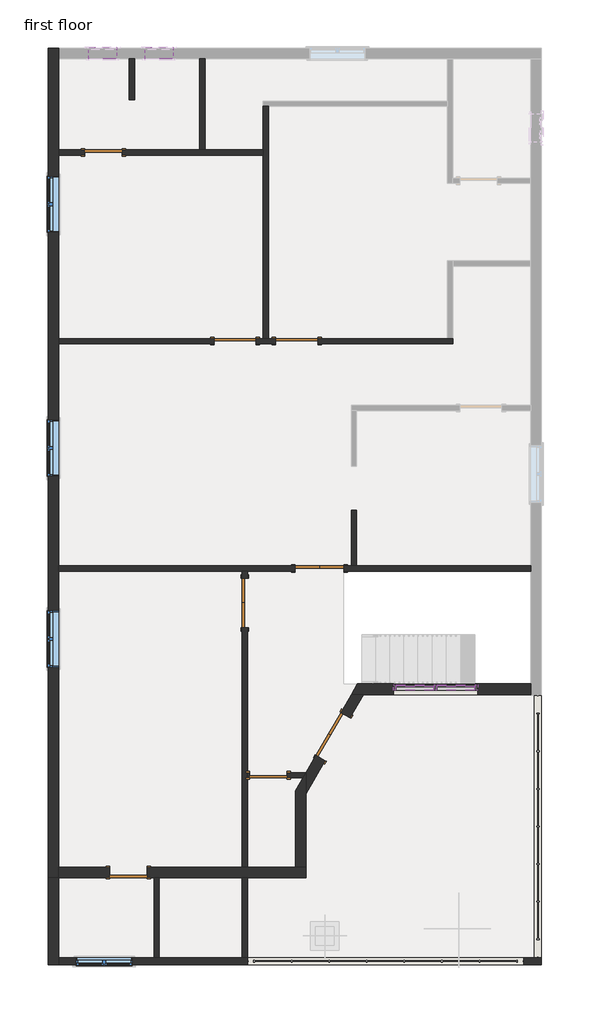
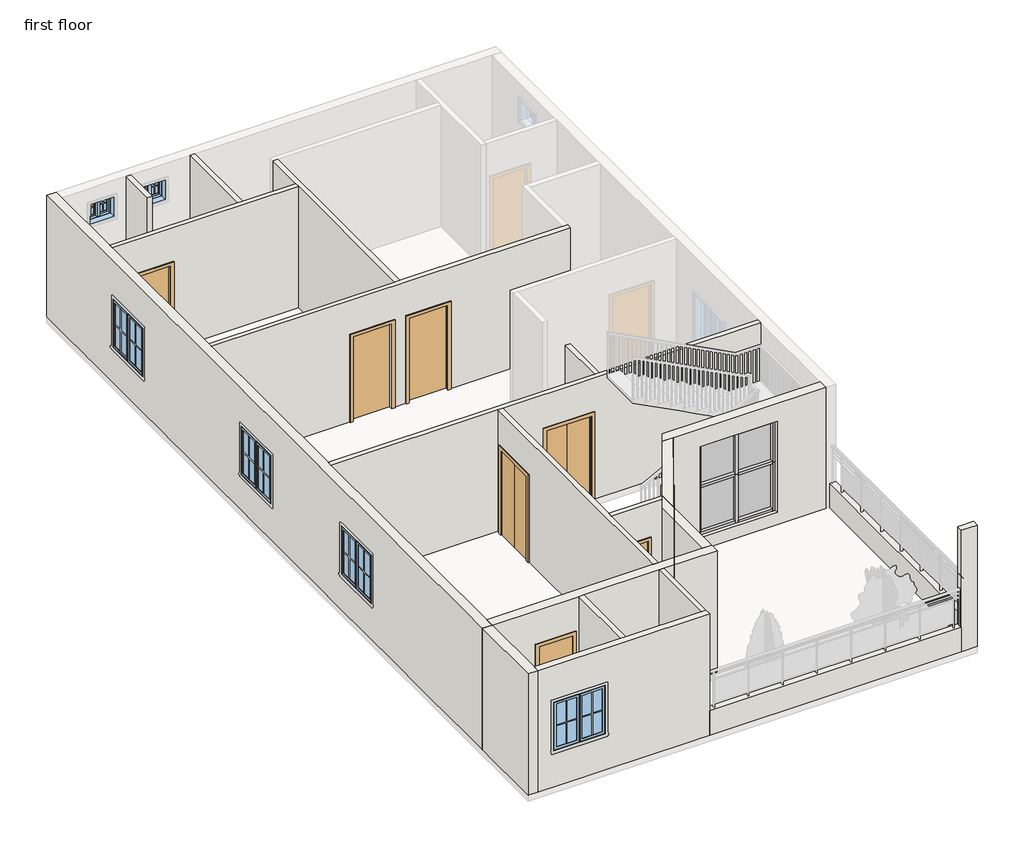
# One storey, part 1 of 4: 21 walls, 12 members, 8 doors, 6 windows, 4 plates.
"""IFC4 building model written with IfcOpenShell, lengths in millimetres."""

from ifc_helpers import new_model, si_unit, frame, origin, place, context, project, spatial, polyline, outline, extrude, faceted_brep, transform, mapped, element, save
from components import door_d52489d9, door_d57fbbae, door_38851409, door_7b345704, single_flush_3_x7_e5f9f3c4, single_flush_3_x7_305aa2a5, member_c17f1be2, member_ad567e07, member_2b49869a, member_a715cb85, member_75074519, member_c4de40ee, system_panel_glazed_f4fd55f0, system_panel_glazed_231200ce, window_79894727, window_casement_double_4_x4_af3140d2, window_casement_double_4_x4_191d0cfb

model = new_model("IFC4")

# Units and contexts
model_context = context("Model", 3, world=origin())
ifc_project = project(units=[si_unit("LENGTHUNIT", "METRE", prefix="MILLI")], contexts=[model_context])

# Site, building, storey
site = spatial("IfcSite", under=ifc_project)
building = spatial("IfcBuilding", under=site)
storey = spatial("IfcBuildingStorey", under=building, Name="first floor", Elevation=3200.4)

# Doors
placement = place(None, origin())
door_shape = door_d52489d9(model_context)
element("IfcDoor", 1, ObjectType="Door-Double-Flush_Panel : 3'6\"X7'", at=placement, inside=storey, context=model_context, shape_type="MappedRepresentation", body=[
    mapped(door_shape, transform((388.5194418, -4721.06525, 3200.4), x_axis=(0.5010362705417002, 0.8654262854811288, 0.0), y_axis=(-0.8654262854811288, 0.5010362705417002, 0.0), z_axis=(0.0, 0.0, 1.0))),
])
door_2_shape = door_d57fbbae(model_context)
element("IfcDoor", 2, ObjectType="Door-Double-Flush_Panel : 3'6\"X7'", at=placement, inside=storey, context=model_context, shape_type="MappedRepresentation", body=[
    mapped(door_2_shape, transform((96.8585096, -1088.0023906, 3200.4), x_axis=(1.0, 0.0, 0.0), y_axis=(0.0, 1.0, 0.0), z_axis=(0.0, 0.0, 1.0))),
])
element("IfcDoor", 3, ObjectType="Door-Double-Flush_Panel : 3'6\"X7'", at=placement, inside=storey, context=model_context, shape_type="MappedRepresentation", body=[
    mapped(door_2_shape, transform((-1522.3914904, -1830.9523906, 3200.4), x_axis=(0.0, 1.0, 0.0), y_axis=(-1.0, 0.0, 0.0), z_axis=(0.0, 0.0, 1.0))),
])
door_3_shape = door_38851409(model_context)
element("IfcDoor", 4, ObjectType="Single-Flush : 2'8\"X7'", at=placement, inside=storey, context=model_context, shape_type="MappedRepresentation", body=[
    mapped(door_3_shape, transform((-1014.3914904, -5558.4023906, 3200.4), x_axis=(1.0, 0.0, 0.0), y_axis=(0.0, 1.0, 0.0), z_axis=(0.0, 0.0, 1.0))),
])
element("IfcDoor", 5, ObjectType="Single-Flush : 2'8\"X7'", at=placement, inside=storey, context=model_context, shape_type="MappedRepresentation", body=[
    mapped(door_3_shape, transform((-4576.7414904, 7903.5976094, 3200.4), x_axis=(-1.0, 0.0, 0.0), y_axis=(0.0, -1.0, 0.0), z_axis=(0.0, 0.0, 1.0))),
])
door_4_shape = door_7b345704(model_context)
element("IfcDoor", 6, ObjectType="Single-Flush : 2'8\"X7'", at=placement, inside=storey, context=model_context, shape_type="MappedRepresentation", body=[
    mapped(door_4_shape, transform((-4036.9914904, -7660.2523906, 3200.4), x_axis=(1.0, 0.0, 0.0), y_axis=(0.0, 1.0, 0.0), z_axis=(0.0, 0.0, 1.0))),
])
single_flush_3_x7_shape = single_flush_3_x7_e5f9f3c4(model_context)
element("IfcDoor", 7, ObjectType="Single-Flush : 3'X7'", at=placement, inside=storey, context=model_context, shape_type="MappedRepresentation", body=[
    mapped(single_flush_3_x7_shape, transform((-1731.9414904, 3826.8976094, 3200.4), x_axis=(1.0, 0.0, 0.0), y_axis=(0.0, 1.0, 0.0), z_axis=(0.0, 0.0, 1.0))),
])
single_flush_3_x7_2_shape = single_flush_3_x7_305aa2a5(model_context)
element("IfcDoor", 8, ObjectType="Single-Flush : 3'X7'", at=placement, inside=storey, context=model_context, shape_type="MappedRepresentation", body=[
    mapped(single_flush_3_x7_2_shape, transform((-398.4414904, 3826.8976094, 3200.4), x_axis=(-1.0, 0.0, 0.0), y_axis=(0.0, -1.0, 0.0), z_axis=(0.0, 0.0, 1.0))),
])

# Members
member_shape = member_c17f1be2(model_context)
element("IfcMember", 9, ObjectType="Rectangular Mullion : 2.5\" x 5\" rectangular", at=placement, inside=storey, context=model_context, shape_type="MappedRepresentation", body=[
    mapped(member_shape, transform((3456.0085096, -3659.7523906, 5791.2), x_axis=(0.0, 0.0, 1.0), y_axis=(0.0, -1.0, 0.0), z_axis=(1.0, 0.0, 0.0))),
])
element("IfcMember", 10, ObjectType="Rectangular Mullion : 2.5\" x 5\" rectangular", at=placement, inside=storey, context=model_context, shape_type="MappedRepresentation", body=[
    mapped(member_shape, transform((2573.3585096, -3659.7523906, 5791.2), x_axis=(0.0, 0.0, 1.0), y_axis=(0.0, -1.0, 0.0), z_axis=(1.0, 0.0, 0.0))),
])
element("IfcMember", 11, ObjectType="Rectangular Mullion : 2.5\" x 5\" rectangular", at=placement, inside=storey, context=model_context, shape_type="MappedRepresentation", body=[
    mapped(member_shape, transform((1754.2085096, -3659.7523906, 3505.2), x_axis=(0.0, 0.0, -1.0), y_axis=(0.0, -1.0, 0.0), z_axis=(-1.0, 0.0, 0.0))),
])
element("IfcMember", 12, ObjectType="Rectangular Mullion : 2.5\" x 5\" rectangular", at=placement, inside=storey, context=model_context, shape_type="MappedRepresentation", body=[
    mapped(member_shape, transform((2636.8585096, -3659.7523906, 3505.2), x_axis=(0.0, 0.0, -1.0), y_axis=(0.0, -1.0, 0.0), z_axis=(-1.0, 0.0, 0.0))),
])
member_2_shape = member_ad567e07(model_context)
element("IfcMember", 13, ObjectType="Rectangular Mullion : 2.5\" x 5\" rectangular", at=placement, inside=storey, context=model_context, shape_type="MappedRepresentation", body=[
    mapped(member_2_shape, transform((2573.3585096, -3659.7523906, 4724.4), x_axis=(0.0, 0.0, 1.0), y_axis=(0.0, -1.0, 0.0), z_axis=(1.0, 0.0, 0.0))),
])
element("IfcMember", 14, ObjectType="Rectangular Mullion : 2.5\" x 5\" rectangular", at=placement, inside=storey, context=model_context, shape_type="MappedRepresentation", body=[
    mapped(member_2_shape, transform((3456.0085096, -3659.7523906, 4724.4), x_axis=(0.0, 0.0, 1.0), y_axis=(0.0, -1.0, 0.0), z_axis=(1.0, 0.0, 0.0))),
])
member_3_shape = member_2b49869a(model_context)
element("IfcMember", 15, ObjectType="Rectangular Mullion : 2.5\" x 5\" rectangular", at=placement, inside=storey, context=model_context, shape_type="MappedRepresentation", body=[
    mapped(member_3_shape, transform((2605.1085096, -3659.7523906, 3505.2), x_axis=(1.0, 0.0, 0.0), y_axis=(0.0, -1.0, 0.0), z_axis=(0.0, 0.0, -1.0))),
])
member_4_shape = member_a715cb85(model_context)
element("IfcMember", 16, ObjectType="Rectangular Mullion : 2.5\" x 5\" rectangular", at=placement, inside=storey, context=model_context, shape_type="MappedRepresentation", body=[
    mapped(member_4_shape, transform((2605.1085096, -3659.7523906, 4724.4), x_axis=(1.0, 0.0, 0.0), y_axis=(0.0, -1.0, 0.0), z_axis=(0.0, 0.0, -1.0))),
])
member_5_shape = member_75074519(model_context)
element("IfcMember", 17, ObjectType="Rectangular Mullion : 2.5\" x 5\" rectangular", at=placement, inside=storey, context=model_context, shape_type="MappedRepresentation", body=[
    mapped(member_5_shape, transform((3519.5085096, -3659.7523906, 3505.2), x_axis=(1.0, 0.0, 0.0), y_axis=(0.0, -1.0, 0.0), z_axis=(0.0, 0.0, -1.0))),
])
member_6_shape = member_c4de40ee(model_context)
element("IfcMember", 18, ObjectType="Rectangular Mullion : 2.5\" x 5\" rectangular", at=placement, inside=storey, context=model_context, shape_type="MappedRepresentation", body=[
    mapped(member_6_shape, transform((1690.7085096, -3659.7523906, 5791.2), x_axis=(-1.0, 0.0, 0.0), y_axis=(0.0, -1.0, 0.0), z_axis=(0.0, 0.0, 1.0))),
])
element("IfcMember", 19, ObjectType="Rectangular Mullion : 2.5\" x 5\" rectangular", at=placement, inside=storey, context=model_context, shape_type="MappedRepresentation", body=[
    mapped(member_6_shape, transform((3519.5085096, -3659.7523906, 4724.4), x_axis=(1.0, 0.0, 0.0), y_axis=(0.0, -1.0, 0.0), z_axis=(0.0, 0.0, -1.0))),
])
element("IfcMember", 20, ObjectType="Rectangular Mullion : 2.5\" x 5\" rectangular", at=placement, inside=storey, context=model_context, shape_type="MappedRepresentation", body=[
    mapped(member_5_shape, transform((1690.7085096, -3659.7523906, 4724.4), x_axis=(-1.0, 0.0, 0.0), y_axis=(0.0, -1.0, 0.0), z_axis=(0.0, 0.0, 1.0))),
])

# Plates
system_panel_glazed_shape = system_panel_glazed_f4fd55f0(model_context)
element("IfcPlate", 21, ObjectType="System Panel : Glazed", at=placement, inside=storey, context=model_context, shape_type="MappedRepresentation", body=[
    mapped(system_panel_glazed_shape, transform((2163.7835096, -3659.7523906, 4756.15), x_axis=(1.0, 0.0, 0.0), y_axis=(0.0, 1.0, 0.0), z_axis=(0.0, 0.0, 1.0))),
])
element("IfcPlate", 22, ObjectType="System Panel : Glazed", at=placement, inside=storey, context=model_context, shape_type="MappedRepresentation", body=[
    mapped(system_panel_glazed_shape, transform((3046.4335096, -3659.7523906, 4756.15), x_axis=(1.0, 0.0, 0.0), y_axis=(0.0, 1.0, 0.0), z_axis=(0.0, 0.0, 1.0))),
])
system_panel_glazed_2_shape = system_panel_glazed_231200ce(model_context)
element("IfcPlate", 23, ObjectType="System Panel : Glazed", at=placement, inside=storey, context=model_context, shape_type="MappedRepresentation", body=[
    mapped(system_panel_glazed_2_shape, transform((2163.7835096, -3659.7523906, 3568.7), x_axis=(1.0, 0.0, 0.0), y_axis=(0.0, 1.0, 0.0), z_axis=(0.0, 0.0, 1.0))),
])
element("IfcPlate", 24, ObjectType="System Panel : Glazed", at=placement, inside=storey, context=model_context, shape_type="MappedRepresentation", body=[
    mapped(system_panel_glazed_2_shape, transform((3046.4335096, -3659.7523906, 3568.7), x_axis=(1.0, 0.0, 0.0), y_axis=(0.0, 1.0, 0.0), z_axis=(0.0, 0.0, 1.0))),
])

# Walls
element("IfcWall", 25, ObjectType="4.5\"", at=placement, inside=storey, context=model_context, shape_type="Brep", body=[
    faceted_brep([(-5543.5289904, 7846.4476094, 3200.4), (-4983.1414904, 7846.4476094, 3200.4), (-4983.1414904, 7846.4476094, 5334.0), (-4170.3414904, 7846.4476094, 5334.0), (-4170.3414904, 7846.4476094, 3200.4), (-1122.3414904, 7846.4476094, 3200.4), (-1122.3414904, 7846.4476094, 6248.4), (-5543.5289904, 7846.4476094, 6248.4), (-4983.1414904, 7960.7476094, 5334.0), (-4983.1414904, 7960.7476094, 3200.4), (-5543.5289904, 7960.7476094, 3200.4), (-5543.5289904, 7960.7476094, 6248.4), (-2493.9414904, 7960.7476094, 6248.4), (-2379.6414904, 7960.7476094, 6248.4), (-1122.3414904, 7960.7476094, 6248.4), (-1122.3414904, 7960.7476094, 3200.4), (-2379.6414904, 7960.7476094, 3200.4), (-2493.9414904, 7960.7476094, 3200.4), (-4170.3414904, 7960.7476094, 3200.4), (-4170.3414904, 7960.7476094, 5334.0)], [[[0, 1, 2, 3, 4, 5, 6, 7]], [[8, 9, 10, 11, 12, 13, 14, 15, 16, 17, 18, 19]], [[10, 9, 1, 0]], [[18, 17, 16, 15, 5, 4]], [[7, 6, 14, 13, 12, 11]], [[0, 7, 11, 10]], [[6, 5, 15, 14]], [[2, 1, 9, 8]], [[3, 2, 8, 19]], [[4, 3, 19, 18]]]),
])
element("IfcWall", 26, ObjectType="4.5\"", at=placement, inside=storey, context=model_context, shape_type="SweptSolid", body=[
    extrude(outline(polyline([(-2493.9414904, 7960.7476094), (-2493.9414904, 9929.2476094), (-2379.6414904, 9929.2476094), (-2379.6414904, 7960.7476094), (-2493.9414904, 7960.7476094)])), frame((0.0, 0.0, 3200.4), z_axis=(0.0, 0.0, 1.0), x_axis=(1.0, 0.0, 0.0)), (0.0, 0.0, 1.0), 3048.0),
])
element("IfcWall", 27, ObjectType="4.5\"", at=placement, inside=storey, context=model_context, shape_type="SweptSolid", body=[
    extrude(outline(polyline([(-4017.9414904, 9045.2567445), (-4017.9414904, 9929.2476094), (-3903.6414904, 9929.2476094), (-3903.6414904, 9045.2567445), (-4017.9414904, 9045.2567445)])), frame((0.0, 0.0, 3200.4), z_axis=(0.0, 0.0, 1.0), x_axis=(1.0, 0.0, 0.0)), (0.0, 0.0, 1.0), 3048.0),
])
element("IfcWall", 28, ObjectType="4.5\"", at=placement, inside=storey, context=model_context, shape_type="Brep", body=[
    faceted_brep([(-1274.7414904, 3769.7476094, 3200.4), (-855.6414904, 3769.7476094, 3200.4), (-855.6414904, 3769.7476094, 5334.0), (58.7585096, 3769.7476094, 5334.0), (58.7585096, 3769.7476094, 3200.4), (2979.7585096, 3769.7476094, 3200.4), (2979.7585096, 3769.7476094, 6248.4), (-5543.5289904, 3769.7476094, 6248.4), (-5543.5289904, 3769.7476094, 3200.4), (-2189.1414904, 3769.7476094, 3200.4), (-2189.1414904, 3769.7476094, 5334.0), (-1274.7414904, 3769.7476094, 5334.0), (-855.6414904, 3884.0476094, 5334.0), (-855.6414904, 3884.0476094, 3200.4), (-1008.0414904, 3884.0476094, 3200.4), (-1122.3414904, 3884.0476094, 3200.4), (-1274.7414904, 3884.0476094, 3200.4), (-1274.7414904, 3884.0476094, 5334.0), (-2189.1414904, 3884.0476094, 5334.0), (-2189.1414904, 3884.0476094, 3200.4), (-5543.5289904, 3884.0476094, 3200.4), (-5543.5289904, 3884.0476094, 6248.4), (-1122.3414904, 3884.0476094, 6248.4), (-1008.0414904, 3884.0476094, 6248.4), (2865.4585096, 3884.0476094, 6248.4), (2979.7585096, 3884.0476094, 6248.4), (2979.7585096, 3884.0476094, 3200.4), (2865.4585096, 3884.0476094, 3200.4), (58.7585096, 3884.0476094, 3200.4), (58.7585096, 3884.0476094, 5334.0)], [[[0, 1, 2, 3, 4, 5, 6, 7, 8, 9, 10, 11]], [[12, 13, 14, 15, 16, 17, 18, 19, 20, 21, 22, 23, 24, 25, 26, 27, 28, 29]], [[9, 8, 20, 19]], [[28, 27, 26, 5, 4]], [[16, 15, 14, 13, 1, 0]], [[7, 6, 25, 24, 23, 22, 21]], [[8, 7, 21, 20]], [[6, 5, 26, 25]], [[17, 16, 0, 11]], [[18, 17, 11, 10]], [[19, 18, 10, 9]], [[2, 1, 13, 12]], [[3, 2, 12, 29]], [[4, 3, 29, 28]]]),
])
element("IfcWall", 29, ObjectType="4.5\"", at=placement, inside=storey, context=model_context, shape_type="Brep", body=[
    faceted_brep([(4668.8585096, -1145.1523906, 6248.4), (-1465.2414904, -1145.1523906, 6248.4), (-1579.5414904, -1145.1523906, 6248.4), (-5543.5289904, -1145.1523906, 6248.4), (-5543.5289904, -1145.1523906, 3200.4), (-1579.5414904, -1145.1523906, 3200.4), (-1465.2414904, -1145.1523906, 3200.4), (-436.5414904, -1145.1523906, 3200.4), (-436.5414904, -1145.1523906, 5334.0), (630.2585096, -1145.1523906, 5334.0), (630.2585096, -1145.1523906, 3200.4), (4668.8585096, -1145.1523906, 3200.4), (-5543.5289904, -1030.8523906, 6248.4), (782.6585096, -1030.8523906, 6248.4), (896.9585096, -1030.8523906, 6248.4), (4668.8585096, -1030.8523906, 6248.4), (4668.8585096, -1030.8523906, 3200.4), (896.9585096, -1030.8523906, 3200.4), (782.6585096, -1030.8523906, 3200.4), (630.2585096, -1030.8523906, 3200.4), (630.2585096, -1030.8523906, 5334.0), (-436.5414904, -1030.8523906, 5334.0), (-436.5414904, -1030.8523906, 3200.4), (-5543.5289904, -1030.8523906, 3200.4)], [[[0, 1, 2, 3, 4, 5, 6, 7, 8, 9, 10, 11]], [[12, 13, 14, 15, 16, 17, 18, 19, 20, 21, 22, 23]], [[4, 23, 22, 7, 6, 5]], [[16, 11, 10, 19, 18, 17]], [[3, 2, 1, 0, 15, 14, 13, 12]], [[4, 3, 12, 23]], [[0, 11, 16, 15]], [[9, 20, 19, 10]], [[20, 9, 8, 21]], [[21, 8, 7, 22]]]),
])
element("IfcWall", 30, ObjectType="4.5\"", at=placement, inside=storey, context=model_context, shape_type="Brep", body=[
    faceted_brep([(-1579.5414904, -7545.9523906, 6248.4), (-1579.5414904, -1145.1523906, 6248.4), (-1579.5414904, -1145.1523906, 3200.4), (-1579.5414904, -1297.5523906, 3200.4), (-1579.5414904, -1297.5523906, 5334.0), (-1579.5414904, -2364.3523906, 5334.0), (-1579.5414904, -2364.3523906, 3200.4), (-1579.5414904, -7545.9523906, 3200.4), (-1465.2414904, -1145.1523906, 6248.4), (-1465.2414904, -5501.2523906, 6248.4), (-1465.2414904, -5615.5523906, 6248.4), (-1465.2414904, -7545.9523906, 6248.4), (-1465.2414904, -7545.9523906, 3200.4), (-1465.2414904, -5615.5523906, 3200.4), (-1465.2414904, -5501.2523906, 3200.4), (-1465.2414904, -2364.3523906, 3200.4), (-1465.2414904, -2364.3523906, 5334.0), (-1465.2414904, -1297.5523906, 5334.0), (-1465.2414904, -1297.5523906, 3200.4), (-1465.2414904, -1145.1523906, 3200.4)], [[[0, 1, 2, 3, 4, 5, 6, 7]], [[8, 9, 10, 11, 12, 13, 14, 15, 16, 17, 18, 19]], [[2, 19, 18, 3]], [[12, 7, 6, 15, 14, 13]], [[1, 0, 11, 10, 9, 8]], [[0, 7, 12, 11]], [[2, 1, 8, 19]], [[17, 4, 3, 18]], [[4, 17, 16, 5]], [[5, 16, 15, 6]]]),
])
element("IfcWall", 31, ObjectType="4.5\"", at=placement, inside=storey, context=model_context, shape_type="Brep", body=[
    faceted_brep([(-607.9914904, -5615.5523906, 5334.0), (-607.9914904, -5615.5523906, 3200.4), (-261.4151747, -5615.5523906, 3200.4), (-261.4151747, -5615.5523906, 6248.4), (-1465.2414904, -5615.5523906, 6248.4), (-1465.2414904, -5615.5523906, 3200.4), (-1420.7914904, -5615.5523906, 3200.4), (-1420.7914904, -5615.5523906, 5334.0), (-195.2414904, -5501.2523906, 3200.4), (-607.9914904, -5501.2523906, 3200.4), (-607.9914904, -5501.2523906, 5334.0), (-1420.7914904, -5501.2523906, 5334.0), (-1420.7914904, -5501.2523906, 3200.4), (-1465.2414904, -5501.2523906, 3200.4), (-1465.2414904, -5501.2523906, 6248.4), (-195.2414904, -5501.2523906, 6248.4)], [[[0, 1, 2, 3, 4, 5, 6, 7]], [[8, 9, 10, 11, 12, 13, 14, 15]], [[6, 5, 13, 12]], [[2, 1, 9, 8]], [[4, 3, 15, 14]], [[3, 2, 8, 15]], [[5, 4, 14, 13]], [[10, 9, 1, 0]], [[11, 10, 0, 7]], [[12, 11, 7, 6]]]),
])
element("IfcWall", 32, ObjectType="4.5\"", at=placement, inside=storey, context=model_context, shape_type="Brep", body=[
    faceted_brep([(-1122.3414904, 8900.5476094, 3200.4), (-1122.3414904, 7960.7476094, 3200.4), (-1122.3414904, 7846.4476094, 3200.4), (-1122.3414904, 3884.0476094, 3200.4), (-1122.3414904, 3884.0476094, 6248.4), (-1122.3414904, 7846.4476094, 6248.4), (-1122.3414904, 7960.7476094, 6248.4), (-1122.3414904, 8900.5476094, 6248.4), (-1008.0414904, 8900.5476094, 3200.4), (-1008.0414904, 8900.5476094, 6248.4), (-1008.0414904, 3884.0476094, 6248.4), (-1008.0414904, 3884.0476094, 3200.4)], [[[0, 1, 2, 3, 4, 5, 6, 7]], [[8, 9, 10, 11]], [[3, 2, 1, 0, 8, 11]], [[7, 6, 5, 4, 10, 9]], [[0, 7, 9, 8]], [[4, 3, 11, 10]]]),
])
element("IfcWall", 33, ObjectType="4.5\"", at=placement, inside=storey, context=model_context, shape_type="SweptSolid", body=[
    extrude(outline(polyline([(-3484.5414904, -9501.7523906), (-3484.5414904, -7774.5523906), (-3370.2414904, -7774.5523906), (-3370.2414904, -9501.7523906), (-3484.5414904, -9501.7523906)])), frame((0.0, 0.0, 3200.4), z_axis=(0.0, 0.0, 1.0), x_axis=(1.0, 0.0, 0.0)), (0.0, 0.0, 1.0), 3048.0),
])
element("IfcWall", 34, ObjectType="4.5\"", at=placement, inside=storey, context=model_context, shape_type="SweptSolid", body=[
    extrude(outline(polyline([(-1579.5414904, -9501.7523906), (-1579.5414904, -7774.5523906), (-1465.2414904, -7774.5523906), (-1465.2414904, -9501.7523906), (-1579.5414904, -9501.7523906)])), frame((0.0, 0.0, 3200.4), z_axis=(0.0, 0.0, 1.0), x_axis=(1.0, 0.0, 0.0)), (0.0, 0.0, 1.0), 3048.0),
])
element("IfcWall", 35, ObjectType="4.5\"", at=placement, inside=storey, context=model_context, shape_type="SweptSolid", body=[
    extrude(outline(polyline([(782.6585096, -1030.8523906), (782.6585096, 169.2976094), (896.9585096, 169.2976094), (896.9585096, -1030.8523906), (782.6585096, -1030.8523906)])), frame((0.0, 0.0, 3200.4), z_axis=(0.0, 0.0, 1.0), x_axis=(1.0, 0.0, 0.0)), (0.0, 0.0, 1.0), 3048.0),
])
element("IfcWall", 36, ObjectType="6\"", at=placement, inside=storey, context=model_context, shape_type="Brep", body=[
    faceted_brep([(-5543.5289904, -9654.1523906, 3200.4), (-1465.2414904, -9654.1523906, 3200.4), (-1465.2414904, -9654.1523906, 6248.4), (-5543.5289904, -9654.1523906, 6248.4), (-5171.2602404, -9654.1523906, 5334.0), (-3952.0602404, -9654.1523906, 5334.0), (-3952.0602404, -9654.1523906, 4114.8), (-5171.2602404, -9654.1523906, 4114.8), (-5543.5289904, -9501.7523906, 3200.4), (-5543.5289904, -9501.7523906, 6248.4), (-3484.5414904, -9501.7523906, 6248.4), (-3370.2414904, -9501.7523906, 6248.4), (-1579.5414904, -9501.7523906, 6248.4), (-1465.2414904, -9501.7523906, 6248.4), (-1465.2414904, -9501.7523906, 3810.0), (-1465.2414904, -9501.7523906, 3200.4), (-1579.5414904, -9501.7523906, 3200.4), (-3370.2414904, -9501.7523906, 3200.4), (-3484.5414904, -9501.7523906, 3200.4), (-5171.2602404, -9501.7523906, 5334.0), (-5171.2602404, -9501.7523906, 4114.8), (-3952.0602404, -9501.7523906, 4114.8), (-3952.0602404, -9501.7523906, 5334.0)], [[[0, 1, 2, 3], [4, 5, 6, 7]], [[8, 9, 10, 11, 12, 13, 14, 15, 16, 17, 18], [19, 20, 21, 22]], [[1, 0, 8, 18, 17, 16, 15]], [[3, 2, 13, 12, 11, 10, 9]], [[0, 3, 9, 8]], [[20, 19, 4, 7]], [[21, 20, 7, 6]], [[22, 21, 6, 5]], [[19, 22, 5, 4]], [[1, 15, 14, 13, 2]]]),
])
element("IfcWall", 37, ObjectType="6\"", at=placement, inside=storey, context=model_context, shape_type="Brep", body=[
    faceted_brep([(4897.4585096, -9501.7523906, 3200.4), (4745.0585096, -9501.7523906, 3200.4), (4516.4585096, -9501.7523906, 3200.4), (4516.4585096, -9501.7523906, 3810.0), (4516.4585096, -9501.7523906, 6248.4), (4897.4585096, -9501.7523906, 6248.4), (4897.4585096, -9501.7523906, 3810.0), (4897.4585096, -9654.1523906, 3200.4), (4897.4585096, -9654.1523906, 6248.4), (4516.4585096, -9654.1523906, 6248.4), (4516.4585096, -9654.1523906, 3810.0), (4516.4585096, -9654.1523906, 3200.4)], [[[0, 1, 2, 3, 4, 5, 6]], [[7, 8, 9, 10, 11]], [[2, 1, 0, 7, 11]], [[4, 3, 2, 11, 10, 9]], [[5, 4, 9, 8]], [[0, 6, 5, 8, 7]]]),
])
element("IfcWall", 38, ObjectType="6\"", at=placement, inside=storey, context=model_context, shape_type="SweptSolid", body=[
    extrude(outline(polyline([(4745.0585096, -9501.7523906), (4745.0585096, -3824.8523906), (4897.4585096, -3824.8523906), (4897.4585096, -9501.7523906), (4745.0585096, -9501.7523906)])), frame((0.0, 0.0, 3200.4), z_axis=(0.0, 0.0, 1.0), x_axis=(1.0, 0.0, 0.0)), (0.0, 0.0, 1.0), 609.6),
])
element("IfcWall", 39, ObjectType="6\"", at=placement, inside=storey, context=model_context, shape_type="SweptSolid", body=[
    extrude(outline(polyline([(-1465.2414904, -9501.7523906), (4516.4585096, -9501.7523906), (4516.4585096, -9654.1523906), (-1465.2414904, -9654.1523906), (-1465.2414904, -9501.7523906)])), frame((0.0, 0.0, 3200.4), z_axis=(0.0, 0.0, 1.0), x_axis=(1.0, 0.0, 0.0)), (0.0, 0.0, 1.0), 609.6),
])
element("IfcWall", 40, ObjectType="9\" 2", at=placement, inside=storey, context=model_context, shape_type="Brep", body=[
    faceted_brep([(-5772.1289904, 10157.8476094, 3200.4), (-5772.1289904, -7774.5523906, 3200.4), (-5772.1289904, -7774.5523906, 6248.4), (-5772.1289904, 10157.8476094, 6248.4), (-5772.1289904, 7395.5976094, 5334.0), (-5772.1289904, 6176.3976094, 5334.0), (-5772.1289904, 6176.3976094, 4114.8), (-5772.1289904, 7395.5976094, 4114.8), (-5772.1289904, 2125.0976094, 5334.0), (-5772.1289904, 905.8976094, 5334.0), (-5772.1289904, 905.8976094, 4114.8), (-5772.1289904, 2125.0976094, 4114.8), (-5772.1289904, -2002.4023906, 5334.0), (-5772.1289904, -3221.6023906, 5334.0), (-5772.1289904, -3221.6023906, 4114.8), (-5772.1289904, -2002.4023906, 4114.8), (-5543.5289904, 10157.8476094, 3200.4), (-5543.5289904, 10157.8476094, 6248.4), (-5543.5289904, 9929.2476094, 6248.4), (-5543.5289904, 7960.7476094, 6248.4), (-5543.5289904, 7846.4476094, 6248.4), (-5543.5289904, 3884.0476094, 6248.4), (-5543.5289904, 3769.7476094, 6248.4), (-5543.5289904, -1030.8523906, 6248.4), (-5543.5289904, -1145.1523906, 6248.4), (-5543.5289904, -7545.9523906, 6248.4), (-5543.5289904, -7774.5523906, 6248.4), (-5543.5289904, -7774.5523906, 3200.4), (-5543.5289904, -7545.9523906, 3200.4), (-5543.5289904, -1145.1523906, 3200.4), (-5543.5289904, -1030.8523906, 3200.4), (-5543.5289904, 3769.7476094, 3200.4), (-5543.5289904, 3884.0476094, 3200.4), (-5543.5289904, 7846.4476094, 3200.4), (-5543.5289904, 7960.7476094, 3200.4), (-5543.5289904, 9929.2476094, 3200.4), (-5543.5289904, 7395.5976094, 5334.0), (-5543.5289904, 7395.5976094, 4114.8), (-5543.5289904, 6176.3976094, 4114.8), (-5543.5289904, 6176.3976094, 5334.0), (-5543.5289904, 2125.0976094, 5334.0), (-5543.5289904, 2125.0976094, 4114.8), (-5543.5289904, 905.8976094, 4114.8), (-5543.5289904, 905.8976094, 5334.0), (-5543.5289904, -2002.4023906, 5334.0), (-5543.5289904, -2002.4023906, 4114.8), (-5543.5289904, -3221.6023906, 4114.8), (-5543.5289904, -3221.6023906, 5334.0)], [[[0, 1, 2, 3], [4, 5, 6, 7], [8, 9, 10, 11], [12, 13, 14, 15]], [[16, 17, 18, 19, 20, 21, 22, 23, 24, 25, 26, 27, 28, 29, 30, 31, 32, 33, 34, 35], [36, 37, 38, 39], [40, 41, 42, 43], [44, 45, 46, 47]], [[1, 0, 16, 35, 34, 33, 32, 31, 30, 29, 28, 27]], [[3, 2, 26, 25, 24, 23, 22, 21, 20, 19, 18, 17]], [[2, 1, 27, 26]], [[0, 3, 17, 16]], [[37, 36, 4, 7]], [[38, 37, 7, 6]], [[39, 38, 6, 5]], [[36, 39, 5, 4]], [[41, 40, 8, 11]], [[42, 41, 11, 10]], [[43, 42, 10, 9]], [[40, 43, 9, 8]], [[45, 44, 12, 15]], [[46, 45, 15, 14]], [[47, 46, 14, 13]], [[44, 47, 13, 12]]]),
])
element("IfcWall", 41, ObjectType="9\" 2", at=placement, inside=storey, context=model_context, shape_type="Brep", body=[
    faceted_brep([(-3630.5914904, -7774.5523906, 5334.0), (-3630.5914904, -7774.5523906, 3200.4), (-3484.5414904, -7774.5523906, 3200.4), (-3370.2414904, -7774.5523906, 3200.4), (-1579.5414904, -7774.5523906, 3200.4), (-1465.2414904, -7774.5523906, 3200.4), (-195.2414904, -7774.5523906, 3200.4), (-195.2414904, -7774.5523906, 6248.4), (-1465.2414904, -7774.5523906, 6248.4), (-1579.5414904, -7774.5523906, 6248.4), (-3370.2414904, -7774.5523906, 6248.4), (-3484.5414904, -7774.5523906, 6248.4), (-5543.5289904, -7774.5523906, 6248.4), (-5543.5289904, -7774.5523906, 3200.4), (-4443.3914904, -7774.5523906, 3200.4), (-4443.3914904, -7774.5523906, 5334.0), (-195.2414904, -7545.9523906, 3200.4), (-423.8414904, -7545.9523906, 3200.4), (-1465.2414904, -7545.9523906, 3200.4), (-1579.5414904, -7545.9523906, 3200.4), (-3630.5914904, -7545.9523906, 3200.4), (-3630.5914904, -7545.9523906, 5334.0), (-4443.3914904, -7545.9523906, 5334.0), (-4443.3914904, -7545.9523906, 3200.4), (-5543.5289904, -7545.9523906, 3200.4), (-5543.5289904, -7545.9523906, 6248.4), (-1579.5414904, -7545.9523906, 6248.4), (-1465.2414904, -7545.9523906, 6248.4), (-423.8414904, -7545.9523906, 6248.4), (-195.2414904, -7545.9523906, 6248.4)], [[[0, 1, 2, 3, 4, 5, 6, 7, 8, 9, 10, 11, 12, 13, 14, 15]], [[16, 17, 18, 19, 20, 21, 22, 23, 24, 25, 26, 27, 28, 29]], [[14, 13, 24, 23]], [[6, 5, 4, 3, 2, 1, 20, 19, 18, 17, 16]], [[12, 11, 10, 9, 8, 7, 29, 28, 27, 26, 25]], [[13, 12, 25, 24]], [[7, 6, 16, 29]], [[21, 20, 1, 0]], [[22, 21, 0, 15]], [[23, 22, 15, 14]]]),
])
element("IfcWall", 42, ObjectType="9\" 2", at=placement, inside=storey, context=model_context, shape_type="Brep", body=[
    faceted_brep([(-195.2414904, -7545.9523906, 3200.4), (-195.2414904, -5957.5067846, 3200.4), (-195.2414904, -5501.2523906, 3200.4), (-195.2414904, -5501.2523906, 6248.4), (-195.2414904, -5957.5067846, 6248.4), (-195.2414904, -7545.9523906, 6248.4), (-423.8414904, -7545.9523906, 3200.4), (-423.8414904, -7545.9523906, 6248.4), (-423.8414904, -5896.106936, 6248.4), (-423.8414904, -5896.106936, 3200.4)], [[[0, 1, 2, 3, 4, 5]], [[6, 7, 8, 9]], [[2, 1, 0, 6, 9]], [[5, 4, 3, 8, 7]], [[0, 5, 7, 6]], [[3, 2, 9, 8]]]),
])
element("IfcWall", 43, ObjectType="9\" 2", at=placement, inside=storey, context=model_context, shape_type="Brep", body=[
    faceted_brep([(4668.8585096, -3583.5523906, 3200.4), (915.005878, -3583.5523906, 3200.4), (915.005878, -3583.5523906, 6248.4), (4668.8585096, -3583.5523906, 6248.4), (1690.7085096, -3583.5523906, 5791.2), (1690.7085096, -3583.5523906, 3505.2), (3519.5085096, -3583.5523906, 3505.2), (3519.5085096, -3583.5523906, 5791.2), (782.6585096, -3812.1523906, 3200.4), (1046.8057903, -3812.1523906, 3200.4), (4668.8585096, -3812.1523906, 3200.4), (4668.8585096, -3812.1523906, 6248.4), (1046.8057903, -3812.1523906, 6248.4), (782.6585096, -3812.1523906, 6248.4), (1690.7085096, -3812.1523906, 3505.2), (1690.7085096, -3812.1523906, 5791.2), (3519.5085096, -3812.1523906, 5791.2), (3519.5085096, -3812.1523906, 3505.2)], [[[0, 1, 2, 3], [4, 5, 6, 7]], [[8, 9, 10, 11, 12, 13], [14, 15, 16, 17]], [[1, 0, 10, 9, 8]], [[3, 2, 13, 12, 11]], [[0, 3, 11, 10]], [[2, 1, 8, 13]], [[14, 5, 4, 15]], [[15, 4, 7, 16]], [[16, 7, 6, 17]], [[5, 14, 17, 6]]]),
])
element("IfcWall", 44, ObjectType="9\" 2", at=placement, inside=storey, context=model_context, shape_type="Brep", body=[
    faceted_brep([(-195.2414904, -5501.2523906, 6248.4), (782.6585096, -3812.1523906, 6248.4), (782.6585096, -3812.1523906, 3200.4), (556.8539641, -4202.1784236, 3200.4), (556.8539641, -4202.1784236, 5334.0), (22.3484707, -5125.415185, 5334.0), (22.3484707, -5125.415185, 3200.4), (-195.2414904, -5501.2523906, 3200.4), (1046.8057903, -3812.1523906, 6248.4), (-195.2414904, -5957.5067846, 6248.4), (-195.2414904, -5957.5067846, 3200.4), (220.1849195, -5239.9520764, 3200.4), (220.1849195, -5239.9520764, 5334.0), (754.6904129, -4316.7153151, 5334.0), (754.6904129, -4316.7153151, 3200.4), (1046.8057903, -3812.1523906, 3200.4)], [[[0, 1, 2, 3, 4, 5, 6, 7]], [[8, 9, 10, 11, 12, 13, 14, 15]], [[2, 15, 14, 3]], [[10, 7, 6, 11]], [[1, 0, 9, 8]], [[2, 1, 8, 15]], [[0, 7, 10, 9]], [[13, 4, 3, 14]], [[4, 13, 12, 5]], [[5, 12, 11, 6]]]),
])
element("IfcWall", 45, ObjectType="9\" 2", at=placement, inside=storey, context=model_context, shape_type="Brep", body=[
    faceted_brep([(-5772.1289904, -7774.5523906, 3200.4), (-5772.1289904, -9654.1523906, 3200.4), (-5772.1289904, -9654.1523906, 6248.4), (-5772.1289904, -7774.5523906, 6248.4), (-5543.5289904, -7774.5523906, 3200.4), (-5543.5289904, -7774.5523906, 6248.4), (-5543.5289904, -9501.7523906, 6248.4), (-5543.5289904, -9654.1523906, 6248.4), (-5543.5289904, -9654.1523906, 3200.4), (-5543.5289904, -9501.7523906, 3200.4)], [[[0, 1, 2, 3]], [[4, 5, 6, 7, 8, 9]], [[1, 0, 4, 9, 8]], [[3, 2, 7, 6, 5]], [[0, 3, 5, 4]], [[2, 1, 8, 7]]]),
])

# Windows
window_shape = window_79894727(model_context)
element("IfcWindow", 46, ObjectType="Window-Casement-Double : 2'X1'9\"", at=placement, inside=storey, context=model_context, shape_type="MappedRepresentation", body=[
    mapped(window_shape, transform((-4595.7914904, 10043.5476094, 3200.4), x_axis=(1.0, 0.0, 0.0), y_axis=(0.0, 1.0, 0.0), z_axis=(0.0, 0.0, 1.0))),
])
element("IfcWindow", 47, ObjectType="Window-Casement-Double : 2'X1'9\"", at=placement, inside=storey, context=model_context, shape_type="MappedRepresentation", body=[
    mapped(window_shape, transform((-3376.5914904, 10043.5476094, 3200.4), x_axis=(1.0, 0.0, 0.0), y_axis=(0.0, 1.0, 0.0), z_axis=(0.0, 0.0, 1.0))),
])
window_casement_double_4_x4_shape = window_casement_double_4_x4_af3140d2(model_context)
element("IfcWindow", 48, ObjectType="Window-Casement-Double : 4'X4'", at=placement, inside=storey, context=model_context, shape_type="MappedRepresentation", body=[
    mapped(window_casement_double_4_x4_shape, transform((-5657.8289904, 6785.9976094, 3200.4), x_axis=(0.0, 1.0, 0.0), y_axis=(-1.0, 0.0, 0.0), z_axis=(0.0, 0.0, 1.0))),
])
element("IfcWindow", 49, ObjectType="Window-Casement-Double : 4'X4'", at=placement, inside=storey, context=model_context, shape_type="MappedRepresentation", body=[
    mapped(window_casement_double_4_x4_shape, transform((-5657.8289904, 1515.4976094, 3200.4), x_axis=(0.0, 1.0, 0.0), y_axis=(-1.0, 0.0, 0.0), z_axis=(0.0, 0.0, 1.0))),
])
element("IfcWindow", 50, ObjectType="Window-Casement-Double : 4'X4'", at=placement, inside=storey, context=model_context, shape_type="MappedRepresentation", body=[
    mapped(window_casement_double_4_x4_shape, transform((-5657.8289904, -2612.0023906, 3200.4), x_axis=(0.0, 1.0, 0.0), y_axis=(-1.0, 0.0, 0.0), z_axis=(0.0, 0.0, 1.0))),
])
window_casement_double_4_x4_2_shape = window_casement_double_4_x4_191d0cfb(model_context)
element("IfcWindow", 51, ObjectType="Window-Casement-Double : 4'X4'", at=placement, inside=storey, context=model_context, shape_type="MappedRepresentation", body=[
    mapped(window_casement_double_4_x4_2_shape, transform((-4561.6602404, -9577.9523906, 3200.4), x_axis=(-1.0, 0.0, 0.0), y_axis=(0.0, -1.0, 0.0), z_axis=(0.0, 0.0, 1.0))),
])

save(model, "model.ifc")

# Revit data of these elements
# Type "Door-Double-Flush_Panel : 3'6\"X7'"
#   Type Mark = "12"
#   Construction Type Id = "DOOR"
#   Assembly Code = "C1020"
#   Analytic Construction = "Wooden"
#   Thickness = 0' - 2"
#   Thermal Resistance (R) = 2.5876 (h·ft²·°F)/BTU
#   Swing Angle [instance default] = 90.00°
#   Panel Width = 1' - 9"
#   Heat Transfer Coefficient (U) = 0.3865 BTU/(h·ft²·°F)
#   Height = 7' - 0"
#   Trim Projection Ext = 0' - 1"
#   Trim Projection Int = 0' - 1"
#   Trim Width = 0' - 3"
#   Width = 3' - 6"
#   Define Thermal Properties by = 1
#   Panel Material = Wood - Birch - Solid Stained Light Low Gloss
#   Trim Material = Paint - Sienna
#   Visual Light Transmittance = 0
#   Solar Heat Gain Coefficient = 0
#   Function = (empty or 0)
#   Wall Closure = (empty or 0)
# Type "Single-Flush : 2'8\"X7'"
#   Type Mark = "9"
#   Construction Type Id = "MDOOR"
#   Assembly Code = "C1020"
#   Analytic Construction = "Metal"
#   Thickness = 0' - 2"
#   Heat Transfer Coefficient (U) = 0.651978 BTU/(h·ft²·°F)
#   Height = 7' - 0"
#   Trim Projection Ext = 0' - 1"
#   Trim Projection Int = 0' - 1"
#   Trim Width = 0' - 3"
#   Width = 2' - 8"
#   Define Thermal Properties by = 1
#   Door Material = Door - Panel
#   Frame Material = Door - Frame
#   Visual Light Transmittance = 0
#   Solar Heat Gain Coefficient = 0
#   Function = (empty or 0)
#   Wall Closure = (empty or 0)
# Type "Single-Flush : 3'X7'"
#   Type Mark = "8"
#   Construction Type Id = "MDOOR"
#   Assembly Code = "C1020"
#   Analytic Construction = "Metal"
#   Thickness = 0' - 2"
#   Heat Transfer Coefficient (U) = 0.651978 BTU/(h·ft²·°F)
#   Height = 7' - 0"
#   Trim Projection Ext = 0' - 1"
#   Trim Projection Int = 0' - 1"
#   Trim Width = 0' - 3"
#   Width = 3' - 0"
#   Define Thermal Properties by = 1
#   Door Material = Door - Panel
#   Frame Material = Door - Frame
#   Visual Light Transmittance = 0
#   Solar Heat Gain Coefficient = 0
#   Function = (empty or 0)
#   Wall Closure = (empty or 0)
# Type "Rectangular Mullion : 2.5\" x 5\" rectangular"
#   built-in parameter 1007304 = 0.416667 (stored number, unit not read)
#   built-in parameter 1007301 = 0.104167 (stored number, unit not read)
#   built-in parameter 1007300 = 0.104167 (stored number, unit not read)
# Type "System Panel : Glazed"
#   Construction Type Id = "GSP4R"
#   Analytic Construction = "1/8 in Pilkington single glazing"
#   Visual Light Transmittance = 0.9
#   Solar Heat Gain Coefficient = 0.86
#   Heat Transfer Coefficient (U) = 1.18115 BTU/(h·ft²·°F)
#   Define Thermal Properties by = 1
# Type "4.5\""
#   Assembly Code = "B2010"
#   Layers, outside or top first: 0' - 4 1/2" no material (function 1)
# Type "6\""
#   Assembly Code = "B2010"
#   Layers, outside or top first: 0' - 6" "wall 2" (function 1)
# Type "9\" 2"
#   Assembly Code = "B2010"
#   Layers, outside or top first: 0' - 9" "wall" (function 1)
# Type "Window-Casement-Double : 2'X1'9\""
#   Type Mark = "20"
#   Fire Rating = "0.5h"
#   Assembly Code = "B2020100"
#   Analytic Construction = "Double glazing - domestic"
#   Frame Extension [instance default] = 0' - 0 1/4"
#   Window Inset [instance default] = 0' - 0"
#   Wall Thickness [instance default] = 0' - 6"
#   Interior Wall Closure [instance default] = 0' - 2 1/4"
#   Half Width = 1' - 0"
#   Visual Light Transmittance = 0.81
#   Thermal Resistance (R) = 1.8146 (h·ft²·°F)/BTU
#   Solar Heat Gain Coefficient = 0.76
#   Rough Width = 2' - 0 1/2"
#   Rough Height = 1' - 9 1/2"
#   Height = 1' - 9"
#   Heat Transfer Coefficient (U) = 0.5511 BTU/(h·ft²·°F)
#   Exterior Wall Closure [instance default] = 0' - 1 1/4"
#   Extension Jamb [instance default] = 0' - 2 1/4"
#   Default Sill Height = 7' - 0"
#   Width = 2' - 0"
#   Muntin Visibility = yes
#   Interior Trim Visibility [instance default] = yes
#   Exterior Trim Visibility [instance default] = yes
#   Extension Jamb Visibility [instance default] = yes
#   Interior Trim Material = Wood - Stained
#   Muntin Pattern = Muntin Pattern_2x2 : Muntin Pattern_2x2
#   Interior Trim = Trim-Window-Interior-Flat : Picture Frame
#   Interior Frame Material = Wood - Stained
#   Glass Panel Material = Glass
#   Exterior Trim Material = Clad - White
#   Exterior Trim = Trim-Window-Exterior-Flat : with Sill
#   Exterior Frame Material = Clad - White
#   Wall Closure = (empty or 0)
# Type "Window-Casement-Double : 4'X4'"
#   Type Mark = "19"
#   Fire Rating = "0.5h"
#   Assembly Code = "B2020100"
#   Analytic Construction = "Double glazing - domestic"
#   Frame Extension [instance default] = 0' - 0 1/4"
#   Window Inset [instance default] = 0' - 0"
#   Wall Thickness [instance default] = 0' - 6"
#   Interior Wall Closure [instance default] = 0' - 2 1/4"
#   Half Width = 2' - 0"
#   Visual Light Transmittance = 0.81
#   Thermal Resistance (R) = 1.8146 (h·ft²·°F)/BTU
#   Solar Heat Gain Coefficient = 0.76
#   Rough Width = 4' - 0 1/2"
#   Rough Height = 4' - 0 1/2"
#   Height = 4' - 0"
#   Heat Transfer Coefficient (U) = 0.5511 BTU/(h·ft²·°F)
#   Exterior Wall Closure [instance default] = 0' - 1 1/4"
#   Extension Jamb [instance default] = 0' - 2 1/4"
#   Default Sill Height = 3' - 0"
#   Width = 4' - 0"
#   Muntin Visibility = yes
#   Interior Trim Visibility [instance default] = yes
#   Exterior Trim Visibility [instance default] = yes
#   Extension Jamb Visibility [instance default] = yes
#   Interior Trim Material = Wood - Stained
#   Muntin Pattern = Muntin Pattern_2x2 : Muntin Pattern_2x2
#   Interior Trim = Trim-Window-Interior-Flat : Picture Frame
#   Interior Frame Material = Wood - Stained
#   Glass Panel Material = Glass
#   Exterior Trim Material = Clad - White
#   Exterior Trim = Trim-Window-Exterior-Flat : with Sill
#   Exterior Frame Material = Clad - White
#   Wall Closure = (empty or 0)
# Elements 1, 2, 3 (IfcDoor, "Door-Double-Flush_Panel : 3'6\"X7'")
#   Swing Angle = 90.00°
#   Phase Created = New Construction
#   Materials on its faces: "Paint - Sienna", "Wood - Birch - Solid Stained Light Low Gloss"
# Elements 4, 5, 6 (IfcDoor, "Single-Flush : 2'8\"X7'")
#   Phase Created = New Construction
#   Materials on its faces: "Door - Frame", "Door - Panel"
# Elements 7, 8 (IfcDoor, "Single-Flush : 3'X7'")
#   Phase Created = New Construction
#   Materials on its faces: "Door - Frame", "Door - Panel"
# Elements 9, 10, 11, 12, 13, 14, 15, 16, 17, 18, 19, 20 (IfcMember, "Rectangular Mullion : 2.5\" x 5\" rectangular")
#   Phase Created = New Construction
#   Materials on its faces: "Aluminum"
# Elements 21, 22, 23, 24 (IfcPlate, "System Panel : Glazed")
#   Phase Created = New Construction
#   Materials on its faces: "Glass"
# Elements 25, 26, 27, 28, 29, 30, 31, 32, 33, 35 (IfcWall, "4.5\"")
#   Top Offset = -0' - 6"
#   Base Offset = 0' - 0"
#   wall height = 10' - 0"
#   Phase Created = New Construction
#   Base Constraint = first floor
#   Top Constraint = second floor
#   Materials on its faces: "Default Wall"
# Element 34 (IfcWall, "4.5\"")
#   Top Offset = -0' - 6"
#   Base Offset = 0' - 0"
#   wall height = 10' - 0"
#   Phase Created = New Construction
#   Base Constraint = first floor
#   Top Constraint = second floor
#   Materials on its faces: "Default Wall", "wall 1"
# Element 36 (IfcWall, "6\"")
#   Top Offset = -0' - 6"
#   Base Offset = 0' - 0"
#   wall height = 10' - 0"
#   Phase Created = New Construction
#   Base Constraint = first floor
#   Top Constraint = second floor
#   Materials on its faces: "wall 2", "6\" wall", "wall 1"
# Element 37 (IfcWall, "6\"")
#   Top Offset = -0' - 6"
#   Base Offset = 0' - 0"
#   wall height = 10' - 0"
#   Phase Created = New Construction
#   Base Constraint = first floor
#   Top Constraint = second floor
#   Materials on its faces: "wall 2"
# Elements 38, 39 (IfcWall, "6\"")
#   Top Offset = -0' - 6"
#   Base Offset = 0' - 0"
#   Unconnected Height = 2' - 0"
#   wall height = 2' - 0"
#   Phase Created = New Construction
#   Base Constraint = first floor
#   Materials on its faces: "wall 2"
# Elements 40, 41 (IfcWall, "9\" 2")
#   Top Offset = -0' - 6"
#   Base Offset = 0' - 0"
#   wall height = 10' - 0"
#   Phase Created = New Construction
#   Base Constraint = first floor
#   Top Constraint = second floor
#   Materials on its faces: "wall", "6\" wall", "wall 1"
# Elements 42, 43 (IfcWall, "9\" 2")
#   Top Offset = -0' - 6"
#   Base Offset = 0' - 0"
#   wall height = 10' - 0"
#   Phase Created = New Construction
#   Base Constraint = first floor
#   Top Constraint = second floor
#   Materials on its faces: "wall", "wall 1"
# Element 44 (IfcWall, "9\" 2")
#   Top Offset = -0' - 6"
#   Base Offset = 0' - 0"
#   wall height = 10' - 0"
#   Phase Created = New Construction
#   Base Constraint = first floor
#   Top Constraint = second floor
#   Materials on its faces: "wall", "6\" wall"
# Element 45 (IfcWall, "9\" 2")
#   Top Offset = -0' - 6"
#   Base Offset = 0' - 0"
#   wall height = 10' - 0"
#   Phase Created = New Construction
#   Base Constraint = first floor
#   Top Constraint = second floor
#   Materials on its faces: "wall", "wall 1", "6\" wall"
# Element 46 (IfcWindow, "Window-Casement-Double : 2'X1'9\"")
#   Mark = "14"
#   Window Inset = 0' - 0"
#   Interior Wall Closure = 0' - 2 1/4"
#   Frame Extension = 0' - 0 1/4"
#   Exterior Wall Closure = 0' - 1 1/4"
#   Interior Trim Visibility = yes
#   Exterior Trim Visibility = yes
#   Phase Created = New Construction
#   Materials on its faces: "Wood - Stained", "Glass", "Clad - White"
# Element 47 (IfcWindow, "Window-Casement-Double : 2'X1'9\"")
#   Mark = "15"
#   Window Inset = 0' - 0"
#   Interior Wall Closure = 0' - 2 1/4"
#   Frame Extension = 0' - 0 1/4"
#   Exterior Wall Closure = 0' - 1 1/4"
#   Interior Trim Visibility = yes
#   Exterior Trim Visibility = yes
#   Phase Created = New Construction
#   Materials on its faces: "Wood - Stained", "Glass", "Clad - White"
# Element 48 (IfcWindow, "Window-Casement-Double : 4'X4'")
#   Mark = "10"
#   Window Inset = 0' - 0"
#   Interior Wall Closure = 0' - 2 1/4"
#   Frame Extension = 0' - 0 1/4"
#   Exterior Wall Closure = 0' - 1 1/4"
#   Interior Trim Visibility = yes
#   Exterior Trim Visibility = yes
#   Phase Created = New Construction
#   Materials on its faces: "Wood - Stained", "Glass", "Clad - White"
# Element 49 (IfcWindow, "Window-Casement-Double : 4'X4'")
#   Mark = "11"
#   Window Inset = 0' - 0"
#   Interior Wall Closure = 0' - 2 1/4"
#   Frame Extension = 0' - 0 1/4"
#   Exterior Wall Closure = 0' - 1 1/4"
#   Interior Trim Visibility = yes
#   Exterior Trim Visibility = yes
#   Phase Created = New Construction
#   Materials on its faces: "Wood - Stained", "Glass", "Clad - White"
# Element 50 (IfcWindow, "Window-Casement-Double : 4'X4'")
#   Mark = "12"
#   Window Inset = 0' - 0"
#   Interior Wall Closure = 0' - 2 1/4"
#   Frame Extension = 0' - 0 1/4"
#   Exterior Wall Closure = 0' - 1 1/4"
#   Interior Trim Visibility = yes
#   Exterior Trim Visibility = yes
#   Phase Created = New Construction
#   Materials on its faces: "Wood - Stained", "Glass", "Clad - White"
# Element 51 (IfcWindow, "Window-Casement-Double : 4'X4'")
#   Mark = "17"
#   Window Inset = 0' - 0"
#   Interior Wall Closure = 0' - 2 1/4"
#   Frame Extension = 0' - 0 1/4"
#   Exterior Wall Closure = 0' - 1 1/4"
#   Interior Trim Visibility = yes
#   Exterior Trim Visibility = yes
#   Phase Created = New Construction
#   Materials on its faces: "Wood - Stained", "Glass", "Clad - White"
# Materials
#   "Wood - Birch - Solid Stained Light Low Gloss": class "Wood", colour RGB 210 159 95, transparency 0, Cost = 0
#   "Paint - Sienna": colour RGB 118 70 51, transparency 0, Cost = 0
#   "Door - Panel": class "Wood", colour RGB 210 159 95, transparency 0, Cost = 0
#   "Door - Frame": colour RGB 118 70 51, transparency 0, Cost = 0
#   "wall 2": class "Generic", colour RGB 34 30 27, transparency 0, Cost = 0
#   "wall": class "Generic", colour RGB 93 108 103, transparency 0, Cost = 0
#   "Wood - Stained": class "Wood", colour RGB 224 178 126, transparency 0, Cost = 0
#   "Glass": class "Glass", colour RGB 0 128 192, transparency 0.75, Description = "Soda Lime Glass", Cost = 0
#   "Clad - White": class "Wood", colour RGB 242 242 238, transparency 0, Cost = 0
#   "Aluminum": class "Metal", colour RGB 247 247 247, transparency 0, Description = "Aluminum 6061", Cost = 0
#   "Default Wall": colour RGB 128 128 128, transparency 0, Cost = 0
#   "wall 1": class "Generic", colour RGB 133 142 137, transparency 0, Cost = 0
#   "6\" wall": class "Generic", colour RGB 136 79 68, transparency 0, Cost = 0
